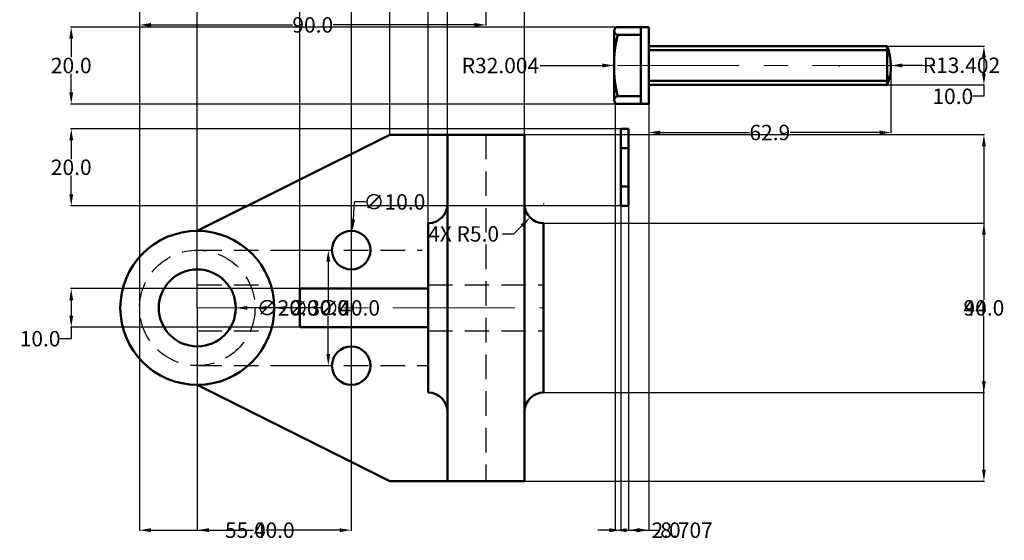
# Model space of a CAD drawing. Units: inches. Extents: x 846 to 1110, y 407 to 675.
# Tile 1 of 2: x 846 to 1102, y 407 to 542. Entities that reach past the tile are written whole.
import ezdxf

# ---------------------------------------------------------------- set-up
doc = ezdxf.new("R2010")
doc.units = ezdxf.units.IN
doc.header["$MEASUREMENT"] = 0
doc.linetypes.add('CENTER', pattern=[50.8, 31.75, -6.35, 6.35, -6.35])
doc.linetypes.add('HIDDEN', pattern=[9.525, 6.35, -3.175])
for name, color, linetype, lineweight in [('M-CNTR', 1, 'CENTER', 18), ('M-DIMS', 2, 'Continuous', 25), ('M-HIDN', 30, 'HIDDEN', 25), ('M-OUTL', 7, 'Continuous', 50)]:
    doc.layers.add(name, color=color, linetype=linetype, lineweight=lineweight)
doc.styles.get("Standard").update_dxf_attribs({"font": 'arial.ttf'})
doc.dimstyles.get("Standard").update_dxf_attribs({"dimtxt": 4, "dimasz": 3, "dimexe": 0.18, "dimexo": 0.0625, "dimgap": 0.09, "dimtad": 0, "dimtih": 1, "dimtoh": 1, "dimdec": 1, "dimzin": 0, "dimdsep": 46, "dimtxsty": 'Standard', "dimcen": 0.09, "dimadec": 0, "dimazin": 0, "dimtfac": 1, "dimtdec": 1, "dimtofl": 0, "dimtmove": 0, "dimatfit": 3, "dimfxl": 1, "dimtolj": 1, "dimtzin": 0, "dimarcsym": 0})

# ---------------------------------------------------------------- blocks, each defined once
blk = doc.blocks.new('*D6')
at = {"layer": 'Defpoints', "color": 0, "transparency": 16777216}
for p in [(877.2, 550.83), (967.2, 550.83), (967.2, 541.12)]:
    blk.add_point(p, dxfattribs=at)
at = {"layer": 'M-DIMS', "color": 0, "lineweight": -2, "transparency": 16777216}
for p, q in [((877.2, 550.77), (877.2, 540.94)), ((967.2, 550.77), (967.2, 540.94)), ((880.2, 541.12), (916.92, 541.12)), ((964.2, 541.12), (927.47, 541.12))]:
    blk.add_line(p, q, dxfattribs=at)
at = {"layer": 'M-DIMS', "color": 0, "transparency": 16777216}
for points in [[(880.2, 541.62), (880.2, 540.62), (877.2, 541.12)], [(964.2, 541.62), (964.2, 540.62), (967.2, 541.12)]]:
    blk.add_solid(points, dxfattribs=at)
at = {"layer": 'M-DIMS', "color": 0, "transparency": 16777216, "insert": (922.2, 541.12), "char_height": 4, "attachment_point": 5}
blk.add_mtext('\\A1;90.0', dxfattribs=at)
blk = doc.blocks.new('*D18')
at = {"layer": 'Defpoints', "color": 0, "transparency": 16777216}
for p in [(932.5, 487.6), (931.89, 477.62)]:
    blk.add_point(p, dxfattribs=at)
at = {"layer": 'M-DIMS', "color": 0, "lineweight": -2, "transparency": 16777216}
for p, q in [((932.97, 495.14), (932.69, 490.59)), ((935.97, 495.14), (932.97, 495.14)), ((932.11, 482.61), (932.29, 482.61)), ((932.2, 482.52), (932.2, 482.7))]:
    blk.add_line(p, q, dxfattribs=at)
at = {"layer": 'M-DIMS', "color": 0, "transparency": 16777216}
blk.add_solid([(932.19, 490.62), (933.19, 490.56), (932.5, 487.6)], dxfattribs=at)
at = {"layer": 'M-DIMS', "color": 0, "transparency": 16777216, "insert": (943.42, 495.14), "char_height": 4, "attachment_point": 5}
blk.add_mtext('\\A1;∅10.0', dxfattribs=at)
blk = doc.blocks.new('*D19')
at = {"layer": 'Defpoints', "color": 0, "transparency": 16777216}
for p in [(917.27, 482.61), (917.27, 452.61), (926.24, 452.61)]:
    blk.add_point(p, dxfattribs=at)
at = {"layer": 'M-DIMS', "color": 0, "lineweight": -2, "transparency": 16777216}
for p, q in [((917.34, 482.61), (926.42, 482.61)), ((926.24, 479.61), (926.24, 469.74)), ((926.24, 455.61), (926.24, 465.47)), ((917.34, 452.61), (926.42, 452.61))]:
    blk.add_line(p, q, dxfattribs=at)
at = {"layer": 'M-DIMS', "color": 0, "transparency": 16777216}
for points in [[(925.74, 479.61), (926.74, 479.61), (926.24, 482.61)], [(925.74, 455.61), (926.74, 455.61), (926.24, 452.61)]]:
    blk.add_solid(points, dxfattribs=at)
at = {"layer": 'M-DIMS', "color": 0, "transparency": 16777216, "insert": (926.24, 467.61), "char_height": 4, "attachment_point": 5}
blk.add_mtext('\\A1;30.0', dxfattribs=at)
blk = doc.blocks.new('*D20')
at = {"layer": 'Defpoints', "color": 0, "transparency": 16777216}
for p in [(1072.42, 530.58), (1009.48, 520.57), (1072.42, 513.17)]:
    blk.add_point(p, dxfattribs=at)
at = {"layer": 'M-DIMS', "color": 0, "lineweight": -2, "transparency": 16777216}
for p, q in [((1072.42, 530.52), (1072.42, 512.99)), ((1009.48, 520.51), (1009.48, 512.99)), ((1012.48, 513.17), (1035.65, 513.17)), ((1069.42, 513.17), (1046.25, 513.17))]:
    blk.add_line(p, q, dxfattribs=at)
at = {"layer": 'M-DIMS', "color": 0, "transparency": 16777216}
for points in [[(1012.48, 513.67), (1012.48, 512.67), (1009.48, 513.17)], [(1069.42, 513.67), (1069.42, 512.67), (1072.42, 513.17)]]:
    blk.add_solid(points, dxfattribs=at)
at = {"layer": 'M-DIMS', "color": 0, "transparency": 16777216, "insert": (1040.95, 513.17), "char_height": 4, "attachment_point": 5}
blk.add_mtext('\\A1;62.9', dxfattribs=at)
blk = doc.blocks.new('*D22')
at = {"layer": 'Defpoints', "color": 0, "transparency": 16777216}
for p in [(942.2, 668.58), (942.2, 512.61), (892.2, 467.61)]:
    blk.add_point(p, dxfattribs=at)
at = {"layer": 'M-DIMS', "color": 0, "lineweight": -2, "transparency": 16777216}
for p, q in [((892.2, 467.67), (892.2, 668.76)), ((895.2, 668.58), (911.92, 668.58)), ((939.2, 668.58), (922.47, 668.58)), ((942.2, 512.67), (942.2, 668.76))]:
    blk.add_line(p, q, dxfattribs=at)
at = {"layer": 'M-DIMS', "color": 0, "transparency": 16777216}
for points in [[(895.2, 669.08), (895.2, 668.08), (892.2, 668.58)], [(939.2, 669.08), (939.2, 668.08), (942.2, 668.58)]]:
    blk.add_solid(points, dxfattribs=at)
at = {"layer": 'M-DIMS', "color": 0, "transparency": 16777216, "insert": (917.2, 668.58), "char_height": 4, "attachment_point": 5}
blk.add_mtext('\\A1;50.0', dxfattribs=at)
blk = doc.blocks.new('*D23')
at = {"layer": 'Defpoints', "color": 0, "transparency": 16777216}
for p in [(957.196639, 668.584955), (942.196639, 512.605991), (957.196639, 512.605991)]:
    blk.add_point(p, dxfattribs=at)
at = {"layer": 'M-DIMS', "color": 0, "lineweight": -2, "transparency": 16777216}
for p, q in [((939.196639, 668.584955), (936.196639, 668.584955)), ((942.196639, 512.668491), (942.196639, 668.764955)), ((957.196639, 512.668491), (957.196639, 668.764955)), ((960.196639, 668.584955), (963.196639, 668.584955))]:
    blk.add_line(p, q, dxfattribs=at)
at = {"layer": 'M-DIMS', "color": 0, "transparency": 16777216}
for points in [[(939.196639, 669.084955), (939.196639, 668.084955), (942.196639, 668.584955)], [(960.196639, 669.084955), (960.196639, 668.084955), (957.196639, 668.584955)]]:
    blk.add_solid(points, dxfattribs=at)
at = {"layer": 'M-DIMS', "color": 0, "transparency": 16777216, "insert": (949.696639, 668.584955), "char_height": 4, "attachment_point": 5}
blk.add_mtext('\\A1;15.0', dxfattribs=at)
blk = doc.blocks.new('*D24')
at = {"layer": 'Defpoints', "color": 0, "transparency": 16777216}
for p in [(977.2, 668.58), (957.2, 512.61), (977.2, 512.61)]:
    blk.add_point(p, dxfattribs=at)
at = {"layer": 'M-DIMS', "color": 0, "lineweight": -2, "transparency": 16777216}
for p, q in [((957.2, 512.67), (957.2, 668.76)), ((960.2, 668.58), (961.88, 668.58)), ((974.2, 668.58), (972.51, 668.58)), ((977.2, 512.67), (977.2, 668.76))]:
    blk.add_line(p, q, dxfattribs=at)
at = {"layer": 'M-DIMS', "color": 0, "transparency": 16777216}
for points in [[(960.2, 669.08), (960.2, 668.08), (957.2, 668.58)], [(974.2, 669.08), (974.2, 668.08), (977.2, 668.58)]]:
    blk.add_solid(points, dxfattribs=at)
at = {"layer": 'M-DIMS', "color": 0, "transparency": 16777216, "insert": (967.2, 668.58), "char_height": 4, "attachment_point": 5}
blk.add_mtext('\\A1;20.0', dxfattribs=at)
blk = doc.blocks.new('*D25')
at = {"layer": 'Defpoints', "color": 0, "transparency": 16777216}
for p in [(892.2, 467.61), (932.2, 452.61), (932.2, 409.86)]:
    blk.add_point(p, dxfattribs=at)
at = {"layer": 'M-DIMS', "color": 0, "lineweight": -2, "transparency": 16777216}
for p, q in [((892.2, 467.54), (892.2, 409.68)), ((932.2, 452.54), (932.2, 409.68)), ((895.2, 409.86), (906.84, 409.86)), ((929.2, 409.86), (917.56, 409.86))]:
    blk.add_line(p, q, dxfattribs=at)
at = {"layer": 'M-DIMS', "color": 0, "transparency": 16777216}
for points in [[(895.2, 410.36), (895.2, 409.36), (892.2, 409.86)], [(929.2, 410.36), (929.2, 409.36), (932.2, 409.86)]]:
    blk.add_solid(points, dxfattribs=at)
at = {"layer": 'M-DIMS', "color": 0, "transparency": 16777216, "insert": (912.2, 409.86), "char_height": 4, "attachment_point": 5}
blk.add_mtext('\\A1;40.0', dxfattribs=at)
blk = doc.blocks.new('*D26')
at = {"layer": 'Defpoints', "color": 0, "transparency": 16777216}
for p in [(952.2, 668.58), (918.81, 472.61), (952.2, 472.61)]:
    blk.add_point(p, dxfattribs=at)
at = {"layer": 'M-DIMS', "color": 0, "lineweight": -2, "transparency": 16777216}
for p, q in [((918.81, 472.67), (918.81, 668.76)), ((921.81, 668.58), (928.66, 668.58)), ((949.2, 668.58), (942.35, 668.58)), ((952.2, 472.67), (952.2, 668.76))]:
    blk.add_line(p, q, dxfattribs=at)
at = {"layer": 'M-DIMS', "color": 0, "transparency": 16777216}
for points in [[(921.81, 669.08), (921.81, 668.08), (918.81, 668.58)], [(949.2, 669.08), (949.2, 668.08), (952.2, 668.58)]]:
    blk.add_solid(points, dxfattribs=at)
at = {"layer": 'M-DIMS', "color": 0, "transparency": 16777216, "insert": (935.51, 668.58), "char_height": 4, "attachment_point": 5}
blk.add_mtext('\\A1;33.38', dxfattribs=at)
blk = doc.blocks.new('*D27')
at = {"layer": 'Defpoints', "color": 0, "transparency": 16777216}
for p in [(918.814083, 472.605991), (859.446639, 462.605991), (918.814083, 462.605991)]:
    blk.add_point(p, dxfattribs=at)
at = {"layer": 'M-DIMS', "color": 0, "lineweight": -2, "transparency": 16777216}
for p, q in [((918.751583, 472.605991), (859.266639, 472.605991)), ((859.446639, 469.605991), (859.446639, 465.605991)), ((918.751583, 462.605991), (859.266639, 462.605991)), ((859.446639, 462.605991), (859.446639, 459.605991)), ((859.446639, 459.605991), (856.446639, 459.605991))]:
    blk.add_line(p, q, dxfattribs=at)
at = {"layer": 'M-DIMS', "color": 0, "transparency": 16777216}
for points in [[(858.946639, 469.605991), (859.946639, 469.605991), (859.446639, 472.605991)], [(858.946639, 465.605991), (859.946639, 465.605991), (859.446639, 462.605991)]]:
    blk.add_solid(points, dxfattribs=at)
at = {"layer": 'M-DIMS', "color": 0, "transparency": 16777216, "insert": (851.356639, 459.605991), "char_height": 4, "attachment_point": 5}
blk.add_mtext('\\A1;10.0', dxfattribs=at)
blk = doc.blocks.new('*D28')
at = {"layer": 'Defpoints', "color": 0, "transparency": 16777216}
for p in [(977.2, 512.61), (977.2, 422.61), (1096.58, 422.61)]:
    blk.add_point(p, dxfattribs=at)
at = {"layer": 'M-DIMS', "color": 0, "lineweight": -2, "transparency": 16777216}
for p, q in [((977.26, 512.61), (1096.76, 512.61)), ((1096.58, 509.61), (1096.58, 469.74)), ((1096.58, 425.61), (1096.58, 465.47)), ((977.26, 422.61), (1096.76, 422.61))]:
    blk.add_line(p, q, dxfattribs=at)
at = {"layer": 'M-DIMS', "color": 0, "transparency": 16777216}
for points in [[(1096.08, 509.61), (1097.08, 509.61), (1096.58, 512.61)], [(1096.08, 425.61), (1097.08, 425.61), (1096.58, 422.61)]]:
    blk.add_solid(points, dxfattribs=at)
at = {"layer": 'M-DIMS', "color": 0, "transparency": 16777216, "insert": (1096.58, 467.61), "char_height": 4, "attachment_point": 5}
blk.add_mtext('\\A1;90.0', dxfattribs=at)
blk = doc.blocks.new('*D29')
at = {"layer": 'Defpoints', "color": 0, "transparency": 16777216}
for p in [(982.2, 489.61), (982.2, 445.61), (1096.58, 445.61)]:
    blk.add_point(p, dxfattribs=at)
at = {"layer": 'M-DIMS', "color": 0, "lineweight": -2, "transparency": 16777216}
for p, q in [((982.26, 489.61), (1096.76, 489.61)), ((1096.58, 486.61), (1096.58, 469.74)), ((1096.58, 448.61), (1096.58, 465.47)), ((982.26, 445.61), (1096.76, 445.61))]:
    blk.add_line(p, q, dxfattribs=at)
at = {"layer": 'M-DIMS', "color": 0, "transparency": 16777216}
for points in [[(1096.08, 486.61), (1097.08, 486.61), (1096.58, 489.61)], [(1096.08, 448.61), (1097.08, 448.61), (1096.58, 445.61)]]:
    blk.add_solid(points, dxfattribs=at)
at = {"layer": 'M-DIMS', "color": 0, "transparency": 16777216, "insert": (1096.58, 467.61), "char_height": 4, "attachment_point": 5}
blk.add_mtext('\\A1;44.0', dxfattribs=at)
blk = doc.blocks.new('*D34')
at = {"layer": 'Defpoints', "color": 0, "transparency": 16777216}
for p in [(877.2, 550.83), (932.2, 550.83), (932.2, 409.86)]:
    blk.add_point(p, dxfattribs=at)
at = {"layer": 'M-DIMS', "color": 0, "lineweight": -2, "transparency": 16777216}
for p, q in [((877.2, 550.77), (877.2, 409.68)), ((932.2, 550.77), (932.2, 409.68)), ((880.2, 409.86), (899.42, 409.86)), ((929.2, 409.86), (909.97, 409.86))]:
    blk.add_line(p, q, dxfattribs=at)
at = {"layer": 'M-DIMS', "color": 0, "transparency": 16777216}
for points in [[(880.2, 410.36), (880.2, 409.36), (877.2, 409.86)], [(929.2, 410.36), (929.2, 409.36), (932.2, 409.86)]]:
    blk.add_solid(points, dxfattribs=at)
at = {"layer": 'M-DIMS', "color": 0, "transparency": 16777216, "insert": (904.7, 409.86), "char_height": 4, "attachment_point": 5}
blk.add_mtext('\\A1;55.0', dxfattribs=at)
blk = doc.blocks.new('*D35')
at = {"layer": 'Defpoints', "color": 0, "transparency": 16777216}
for p in [(1009.48, 540.57), (859.45, 520.57), (1009.48, 520.57)]:
    blk.add_point(p, dxfattribs=at)
at = {"layer": 'M-DIMS', "color": 0, "lineweight": -2, "transparency": 16777216}
for p, q in [((1009.42, 540.57), (859.27, 540.57)), ((859.45, 537.57), (859.45, 532.71)), ((859.45, 523.57), (859.45, 528.44)), ((1009.42, 520.57), (859.27, 520.57))]:
    blk.add_line(p, q, dxfattribs=at)
at = {"layer": 'M-DIMS', "color": 0, "transparency": 16777216}
for points in [[(858.95, 537.57), (859.95, 537.57), (859.45, 540.57)], [(858.95, 523.57), (859.95, 523.57), (859.45, 520.57)]]:
    blk.add_solid(points, dxfattribs=at)
at = {"layer": 'M-DIMS', "color": 0, "transparency": 16777216, "insert": (859.45, 530.57), "char_height": 4, "attachment_point": 5}
blk.add_mtext('\\A1;20.0', dxfattribs=at)
blk = doc.blocks.new('*D36')
at = {"layer": 'Defpoints', "color": 0, "transparency": 16777216}
for p in [(1000.77, 520.87), (1009.48, 520.57), (1009.48, 409.86)]:
    blk.add_point(p, dxfattribs=at)
at = {"layer": 'M-DIMS', "color": 0, "lineweight": -2, "transparency": 16777216}
for p, q in [((1000.77, 520.8), (1000.77, 409.68)), ((1009.48, 520.51), (1009.48, 409.68)), ((1003.77, 409.86), (1006.48, 409.86)), ((1009.48, 409.86), (1012.48, 409.86))]:
    blk.add_line(p, q, dxfattribs=at)
at = {"layer": 'M-DIMS', "color": 0, "transparency": 16777216}
for points in [[(1003.77, 410.36), (1003.77, 409.36), (1000.77, 409.86)], [(1006.48, 410.36), (1006.48, 409.36), (1009.48, 409.86)]]:
    blk.add_solid(points, dxfattribs=at)
at = {"layer": 'M-DIMS', "color": 0, "transparency": 16777216, "insert": (1019.32, 409.86), "char_height": 4, "attachment_point": 5}
blk.add_mtext('\\A1;8.707', dxfattribs=at)
blk = doc.blocks.new('*D37')
at = {"layer": 'Defpoints', "color": 0, "transparency": 16777216}
for p in [(1071.421693, 535.573296), (1071.480881, 525.573296), (1096.581479, 525.573296)]:
    blk.add_point(p, dxfattribs=at)
at = {"layer": 'M-DIMS', "color": 0, "lineweight": -2, "transparency": 16777216}
for p, q in [((1071.484193, 535.573296), (1096.761479, 535.573296)), ((1096.581479, 532.573296), (1096.581479, 528.573296)), ((1071.543381, 525.573296), (1096.761479, 525.573296)), ((1096.581479, 525.573296), (1096.581479, 522.573296)), ((1096.581479, 522.573296), (1093.581479, 522.573296))]:
    blk.add_line(p, q, dxfattribs=at)
at = {"layer": 'M-DIMS', "color": 0, "transparency": 16777216}
for points in [[(1096.081479, 532.573296), (1097.081479, 532.573296), (1096.581479, 535.573296)], [(1096.081479, 528.573296), (1097.081479, 528.573296), (1096.581479, 525.573296)]]:
    blk.add_solid(points, dxfattribs=at)
at = {"layer": 'M-DIMS', "color": 0, "transparency": 16777216, "insert": (1088.491479, 522.573296), "char_height": 4, "attachment_point": 5}
blk.add_mtext('\\A1;10.0', dxfattribs=at)
blk = doc.blocks.new('*D38')
at = {"layer": 'Defpoints', "color": 0, "transparency": 16777216}
for p in [(1002.25, 514.14), (859.45, 494.14), (1002.25, 494.14)]:
    blk.add_point(p, dxfattribs=at)
at = {"layer": 'M-DIMS', "color": 0, "lineweight": -2, "transparency": 16777216}
for p, q in [((1002.19, 514.14), (859.27, 514.14)), ((859.45, 511.14), (859.45, 506.27)), ((859.45, 497.14), (859.45, 502.01)), ((1002.19, 494.14), (859.27, 494.14))]:
    blk.add_line(p, q, dxfattribs=at)
at = {"layer": 'M-DIMS', "color": 0, "transparency": 16777216}
for points in [[(858.95, 511.14), (859.95, 511.14), (859.45, 514.14)], [(858.95, 497.14), (859.95, 497.14), (859.45, 494.14)]]:
    blk.add_solid(points, dxfattribs=at)
at = {"layer": 'M-DIMS', "color": 0, "transparency": 16777216, "insert": (859.45, 504.14), "char_height": 4, "attachment_point": 5}
blk.add_mtext('\\A1;20.0', dxfattribs=at)
blk = doc.blocks.new('*D39')
at = {"layer": 'Defpoints', "color": 0, "transparency": 16777216}
for p in [(1002.25, 494.14), (1004.25, 494.14), (1004.25, 409.86)]:
    blk.add_point(p, dxfattribs=at)
at = {"layer": 'M-DIMS', "color": 0, "lineweight": -2, "transparency": 16777216}
for p, q in [((1002.25, 494.08), (1002.25, 409.68)), ((1004.25, 494.08), (1004.25, 409.68)), ((999.25, 409.86), (996.25, 409.86)), ((1007.25, 409.86), (1010.25, 409.86))]:
    blk.add_line(p, q, dxfattribs=at)
at = {"layer": 'M-DIMS', "color": 0, "transparency": 16777216}
for points in [[(999.25, 410.36), (999.25, 409.36), (1002.25, 409.86)], [(1007.25, 410.36), (1007.25, 409.36), (1004.25, 409.86)]]:
    blk.add_solid(points, dxfattribs=at)
at = {"layer": 'M-DIMS', "color": 0, "transparency": 16777216, "insert": (1014.01, 409.86), "char_height": 4, "attachment_point": 5}
blk.add_mtext('\\A1;2.0', dxfattribs=at)
blk = doc.blocks.new('*D40')
at = {"layer": 'Defpoints', "color": 0, "transparency": 16777216}
for p in [(872.2, 467.61), (912.2, 467.61)]:
    blk.add_point(p, dxfattribs=at)
at = {"layer": 'M-DIMS', "color": 0, "lineweight": -2, "transparency": 16777216}
for p, q in [((892.11, 467.61), (892.29, 467.61)), ((892.2, 467.52), (892.2, 467.7)), ((924.2, 467.61), (915.2, 467.61))]:
    blk.add_line(p, q, dxfattribs=at)
at = {"layer": 'M-DIMS', "color": 0, "transparency": 16777216}
blk.add_solid([(915.2, 468.11), (915.2, 467.11), (912.2, 467.61)], dxfattribs=at)
at = {"layer": 'M-DIMS', "color": 0, "transparency": 16777216, "insert": (931.65, 467.61), "char_height": 4, "attachment_point": 5}
blk.add_mtext('\\A1;∅40.0', dxfattribs=at)
blk = doc.blocks.new('*D41')
at = {"layer": 'Defpoints', "color": 0, "transparency": 16777216}
for p in [(877.2, 467.61), (907.2, 467.61)]:
    blk.add_point(p, dxfattribs=at)
at = {"layer": 'M-DIMS', "color": 0, "lineweight": -2, "transparency": 16777216}
for p, q in [((892.11, 467.61), (892.29, 467.61)), ((892.2, 467.52), (892.2, 467.7)), ((916.2, 467.61), (910.2, 467.61))]:
    blk.add_line(p, q, dxfattribs=at)
at = {"layer": 'M-DIMS', "color": 0, "transparency": 16777216}
blk.add_solid([(910.2, 468.11), (910.2, 467.11), (907.2, 467.61)], dxfattribs=at)
at = {"layer": 'M-DIMS', "color": 0, "transparency": 16777216, "insert": (923.65, 467.61), "char_height": 4, "attachment_point": 5}
blk.add_mtext('\\A1;∅30.0', dxfattribs=at)
blk = doc.blocks.new('*D42')
at = {"layer": 'Defpoints', "color": 0, "transparency": 16777216}
for p in [(882.2, 467.61), (902.2, 467.61)]:
    blk.add_point(p, dxfattribs=at)
at = {"layer": 'M-DIMS', "color": 0, "lineweight": -2, "transparency": 16777216}
for p, q in [((892.11, 467.61), (892.29, 467.61)), ((892.2, 467.52), (892.2, 467.7)), ((908.2, 467.61), (905.2, 467.61))]:
    blk.add_line(p, q, dxfattribs=at)
at = {"layer": 'M-DIMS', "color": 0, "transparency": 16777216}
blk.add_solid([(905.2, 468.11), (905.2, 467.11), (902.2, 467.61)], dxfattribs=at)
at = {"layer": 'M-DIMS', "color": 0, "transparency": 16777216, "insert": (915.65, 467.61), "char_height": 4, "attachment_point": 5}
blk.add_mtext('\\A1;∅20.0', dxfattribs=at)
blk = doc.blocks.new('*D43')
at = {"layer": 'Defpoints', "color": 0, "transparency": 16777216}
for p in [(982.2, 494.61), (978.66, 491.07)]:
    blk.add_point(p, dxfattribs=at)
at = {"layer": 'M-DIMS', "color": 0, "lineweight": -2, "transparency": 16777216}
for p, q in [((982.11, 494.61), (982.29, 494.61)), ((982.2, 494.52), (982.2, 494.7)), ((974.42, 486.83), (976.54, 488.95)), ((971.42, 486.83), (974.42, 486.83))]:
    blk.add_line(p, q, dxfattribs=at)
at = {"layer": 'M-DIMS', "color": 0, "transparency": 16777216}
blk.add_solid([(976.19, 489.3), (976.89, 488.6), (978.66, 491.07)], dxfattribs=at)
at = {"layer": 'M-DIMS', "color": 0, "transparency": 16777216, "insert": (961.4, 486.83), "char_height": 4, "attachment_point": 5}
blk.add_mtext('\\A1;4X R5.0', dxfattribs=at)
blk = doc.blocks.new('*D47')
at = {"layer": 'Defpoints', "color": 0, "transparency": 16777216}
for p in [(1000.46, 530.57), (1032.47, 530.57)]:
    blk.add_point(p, dxfattribs=at)
at = {"layer": 'M-DIMS', "color": 0, "lineweight": -2, "transparency": 16777216}
for p, q in [((981.26, 530.57), (997.46, 530.57)), ((1032.38, 530.57), (1032.56, 530.57)), ((1032.47, 530.48), (1032.47, 530.66))]:
    blk.add_line(p, q, dxfattribs=at)
at = {"layer": 'M-DIMS', "color": 0, "transparency": 16777216}
blk.add_solid([(997.46, 531.07), (997.46, 530.07), (1000.46, 530.57)], dxfattribs=at)
at = {"layer": 'M-DIMS', "color": 0, "transparency": 16777216, "insert": (970.96, 530.57), "char_height": 4, "attachment_point": 5}
blk.add_mtext('\\A1;R32.004', dxfattribs=at)
blk = doc.blocks.new('*D48')
at = {"layer": 'Defpoints', "color": 0, "transparency": 16777216}
for p in [(1059.02, 530.5), (1072.42, 530.58)]:
    blk.add_point(p, dxfattribs=at)
at = {"layer": 'M-DIMS', "color": 0, "lineweight": -2, "transparency": 16777216}
for p, q in [((1058.93, 530.5), (1059.11, 530.5)), ((1059.02, 530.41), (1059.02, 530.59)), ((1080.46, 530.63), (1075.42, 530.6))]:
    blk.add_line(p, q, dxfattribs=at)
at = {"layer": 'M-DIMS', "color": 0, "transparency": 16777216}
blk.add_solid([(1075.42, 531.1), (1075.42, 530.1), (1072.42, 530.58)], dxfattribs=at)
at = {"layer": 'M-DIMS', "color": 0, "transparency": 16777216, "insert": (1090.75, 530.63), "char_height": 4, "attachment_point": 5}
blk.add_mtext('\\A1;R13.402', dxfattribs=at)

msp = doc.modelspace()

# ---------------------------------------------------------------- linework, layer by layer
at = {"layer": 'M-CNTR'}
for p, q in [((892.1966, 462.3642), (892.1966, 565.835)), ((1083.8315, 530.5733), (1000.4809, 530.5733)), ((892.1966, 467.606), (982.1966, 467.606))]:
    msp.add_line(p, q, dxfattribs=at)
at = {"layer": 'M-HIDN'}
for p, q in [((967.1966, 512.606), (967.1966, 422.606)), ((892.1966, 482.606), (950.6476, 482.606)), ((892.1966, 473.606), (911.2754, 473.606)), ((952.1966, 473.606), (982.1966, 473.606)), ((892.1966, 461.606), (911.2754, 461.606)), ((952.1966, 461.606), (982.1966, 461.606)), ((892.1966, 452.606), (951.8976, 452.606))]:
    msp.add_line(p, q, dxfattribs=at)
msp.add_circle((892.1966, 467.606), 15, dxfattribs=at)
at = {"layer": 'M-OUTL'}
for p, q in [((1009.4809, 540.5733), (1001.4809, 540.5733)), ((1007.4809, 520.5733), (1007.4809, 540.5733)), ((1009.4809, 520.5733), (1009.4809, 540.5733)), ((1000.4809, 539.5733), (1000.4809, 521.5733)), ((1001.4809, 538.5733), (1007.4809, 538.5733)), ((1009.4809, 535.5733), (1071.4809, 535.5733)), ((1071.4809, 535.5733), (1071.4809, 525.5733)), ((1009.4809, 534.5733), (1071.7851, 534.5733)), ((1071.8311, 526.5733), (1009.4809, 526.5733)), ((1071.4809, 525.5733), (1009.4809, 525.5733)), ((1007.4809, 522.5733), (1001.4809, 522.5733)), ((1001.4809, 520.5733), (1009.4809, 520.5733)), ((942.1966, 512.606), (892.1966, 487.606)), ((942.1966, 512.606), (977.1966, 512.606)), ((957.1966, 512.606), (957.1966, 422.606)), ((977.1966, 512.606), (977.1966, 422.606)), ((1002.2545, 494.1383), (1002.2545, 514.1383)), ((1004.2545, 514.1383), (1002.2545, 514.1383)), ((1004.2545, 494.1383), (1004.2545, 514.1383)), ((1004.2545, 509.1383), (1002.2545, 509.1383)), ((1002.2545, 499.1383), (1004.2545, 499.1383)), ((1002.2545, 494.1383), (1004.2545, 494.1383)), ((952.1966, 489.606), (952.1966, 445.606)), ((982.1966, 489.606), (982.1966, 445.606)), ((918.8141, 472.606), (918.8141, 462.606)), ((918.8141, 472.606), (952.1966, 472.606)), ((918.8141, 462.606), (952.1966, 462.606)), ((892.1966, 447.606), (942.1966, 422.606)), ((942.1966, 422.606), (977.1966, 422.606))]:
    msp.add_line(p, q, dxfattribs=at)
for centre, radius in [((892.1966, 467.606), 20), ((932.1966, 482.606), 5), ((892.1966, 467.606), 10), ((932.1966, 452.606), 5)]:
    msp.add_circle(centre, radius, dxfattribs=at)
for centre, radius, start, end in [((1001.4809, 539.5733), 1, 90, 270), ((1032.4685, 530.5733), 32.0036, 165.524153, 194.475847), ((1059.0174, 530.4997), 13.4018, 338.432761, 22.24547), ((1001.4809, 521.5733), 1, 90, 270), ((952.1966, 494.606), 5, 270, 0), ((982.1966, 494.606), 5, 180, 270), ((952.1966, 440.606), 5, 0, 90), ((982.1966, 440.606), 5, 90, 180)]:
    msp.add_arc(centre, radius, start, end, dxfattribs=at)

# ---------------------------------------------------------------- dimensions: what is measured, and where the dimension line sits
at = {"layer": 'M-DIMS'}
for base, p1, p2, override, picture, middle in [((942.1966, 668.585), (892.1966, 467.606), (942.1966, 512.606), {"dimdec": 1, "dimlfac": 1, "dimrnd": 0, "dimzin": 0, "dimdsep": 46, "dimlunit": 2}, '*D22', (917.1966, 668.585)), ((952.1966, 668.585), (918.8141, 472.606), (952.1966, 472.606), {"dimdec": 2, "dimlfac": 1, "dimrnd": 0, "dimzin": 0, "dimdsep": 46, "dimlunit": 2}, '*D26', (935.5054, 668.585)), ((957.1966, 668.585), (942.1966, 512.606), (957.1966, 512.606), {"dimdec": 1, "dimlfac": 1, "dimrnd": 0, "dimzin": 0, "dimdsep": 46, "dimlunit": 2}, '*D23', (949.6966, 668.585)), ((977.1966, 668.585), (957.1966, 512.606), (977.1966, 512.606), {"dimdec": 1, "dimlfac": 1, "dimrnd": 0, "dimzin": 0, "dimdsep": 46, "dimlunit": 2}, '*D24', (967.1966, 668.585)), ((967.1966, 541.1223), (877.1966, 550.835), (967.1966, 550.835), {"dimclrd": 0, "dimclre": 0, "dimclrt": 0}, '*D6', (922.1966, 541.1223)), ((932.1966, 409.856), (877.1966, 550.835), (932.1966, 550.835), {"dimdec": 1, "dimlfac": 1, "dimrnd": 0, "dimzin": 0, "dimdsep": 46, "dimlunit": 2}, '*D34', (904.6966, 409.856)), ((1072.4189, 513.1666), (1009.4809, 520.5733), (1072.4189, 530.579), {"dimclrd": 0, "dimclre": 0, "dimclrt": 0}, '*D20', (1040.9499, 513.1666)), ((1009.4809, 409.856), (1000.7738, 520.8662), (1009.4809, 520.5733), {"dimdec": 3, "dimlfac": 1, "dimrnd": 0, "dimzin": 0, "dimdsep": 46, "dimlunit": 2}, '*D36', (1019.3226, 409.856)), ((1004.2545, 409.856), (1002.2545, 494.1383), (1004.2545, 494.1383), {"dimdec": 1, "dimlfac": 1, "dimrnd": 0, "dimzin": 0, "dimdsep": 46, "dimlunit": 2}, '*D39', (1014.0129, 409.856)), ((932.1966, 409.856), (892.1966, 467.606), (932.1966, 452.606), {"dimdec": 1, "dimlfac": 1, "dimrnd": 0, "dimzin": 0, "dimdsep": 46, "dimlunit": 2}, '*D25', (912.1966, 409.856))]:
    dim = msp.add_linear_dim(base=base, p1=p1, p2=p2, dimstyle='Standard', override=override, dxfattribs=at)
    dim.commit()
    dim.dimension.update_dxf_attribs({"geometry": picture, "text_midpoint": middle})
for base, p1, p2, override, picture, middle in [((859.4466, 520.5733), (1009.4809, 540.5733), (1009.4809, 520.5733), {"dimdec": 1, "dimlfac": 1, "dimrnd": 0, "dimzin": 0, "dimdsep": 46, "dimlunit": 2}, '*D35', (859.4466, 530.5733)), ((1096.5815, 525.5733), (1071.4217, 535.5733), (1071.4809, 525.5733), {"dimdec": 1, "dimlfac": 1, "dimrnd": 0, "dimzin": 0, "dimdsep": 46, "dimlunit": 2}, '*D37', (1088.4915, 522.5733)), ((859.4466, 494.1383), (1002.2545, 514.1383), (1002.2545, 494.1383), {"dimdec": 1, "dimlfac": 1, "dimrnd": 0, "dimzin": 0, "dimdsep": 46, "dimlunit": 2}, '*D38', (859.4466, 504.1383)), ((1096.5815, 422.606), (977.1966, 512.606), (977.1966, 422.606), {"dimdec": 1, "dimlfac": 1, "dimrnd": 0, "dimzin": 0, "dimdsep": 46, "dimlunit": 2}, '*D28', (1096.5815, 467.606)), ((1096.5815, 445.606), (982.1966, 489.606), (982.1966, 445.606), {"dimdec": 1, "dimlfac": 1, "dimrnd": 0, "dimzin": 0, "dimdsep": 46, "dimlunit": 2}, '*D29', (1096.5815, 467.606)), ((926.2446, 452.606), (917.2748, 482.606), (917.2748, 452.606), {"dimclrd": 0, "dimclre": 0, "dimclrt": 0}, '*D19', (926.2446, 467.606)), ((859.4466, 462.606), (918.8141, 472.606), (918.8141, 462.606), {"dimdec": 1, "dimlfac": 1, "dimrnd": 0, "dimzin": 0, "dimdsep": 46, "dimlunit": 2}, '*D27', (851.3566, 459.606))]:
    dim = msp.add_linear_dim(base=base, p1=p1, p2=p2, angle=90, dimstyle='Standard', override=override, dxfattribs=at)
    dim.commit()
    dim.dimension.update_dxf_attribs({"geometry": picture, "text_midpoint": middle})
for center, mpoint, picture, middle in [((1032.4685, 530.5733), (1000.4649, 530.573), '*D47', (981.2627, 530.5728)), ((1059.0174, 530.4997), (1072.4189, 530.579), '*D48', (1080.4599, 530.6266))]:
    dim = msp.add_radius_dim(center=center, mpoint=mpoint, dimstyle='Standard', override={"dimdec": 3, "dimlfac": 1, "dimrnd": 0, "dimzin": 0, "dimdsep": 46, "dimlunit": 2}, dxfattribs=at)
    dim.commit()
    dim.dimension.update_dxf_attribs({"geometry": picture, "text_midpoint": middle, "dimtype": 164})
for p1, p2, override, picture, middle in [((931.8889, 477.6155), (932.5044, 487.5965), {"dimclrd": 0, "dimclre": 0, "dimclrt": 0}, '*D18', (943.4238, 495.1395)), ((872.1966, 467.606), (912.1966, 467.606), {"dimdec": 1, "dimlfac": 1, "dimrnd": 0, "dimzin": 0, "dimdsep": 46, "dimlunit": 2}, '*D40', (924.1966, 467.606)), ((877.1966, 467.606), (907.1966, 467.606), {"dimdec": 1, "dimlfac": 1, "dimrnd": 0, "dimzin": 0, "dimdsep": 46, "dimlunit": 2}, '*D41', (916.1966, 467.606)), ((882.1966, 467.606), (902.1966, 467.606), {"dimdec": 1, "dimlfac": 1, "dimrnd": 0, "dimzin": 0, "dimdsep": 46, "dimlunit": 2}, '*D42', (908.1966, 467.606))]:
    dim = msp.add_diameter_dim_2p(p1=p1, p2=p2, dimstyle='Standard', override=override, dxfattribs=at)
    dim.commit()
    dim.dimension.update_dxf_attribs({"geometry": picture, "text_midpoint": middle, "dimtype": 163})
dim = msp.add_radius_dim(center=(982.1966, 494.606), mpoint=(978.6613, 491.0703), text='4X <>', dimstyle='Standard', override={"dimdec": 1, "dimlfac": 1, "dimrnd": 0, "dimzin": 0, "dimdsep": 46, "dimlunit": 2}, dxfattribs=at)
dim.commit()
dim.dimension.update_dxf_attribs({"geometry": '*D43', "text_midpoint": (961.4025, 486.8274)})

doc.saveas('drawing.dxf')
